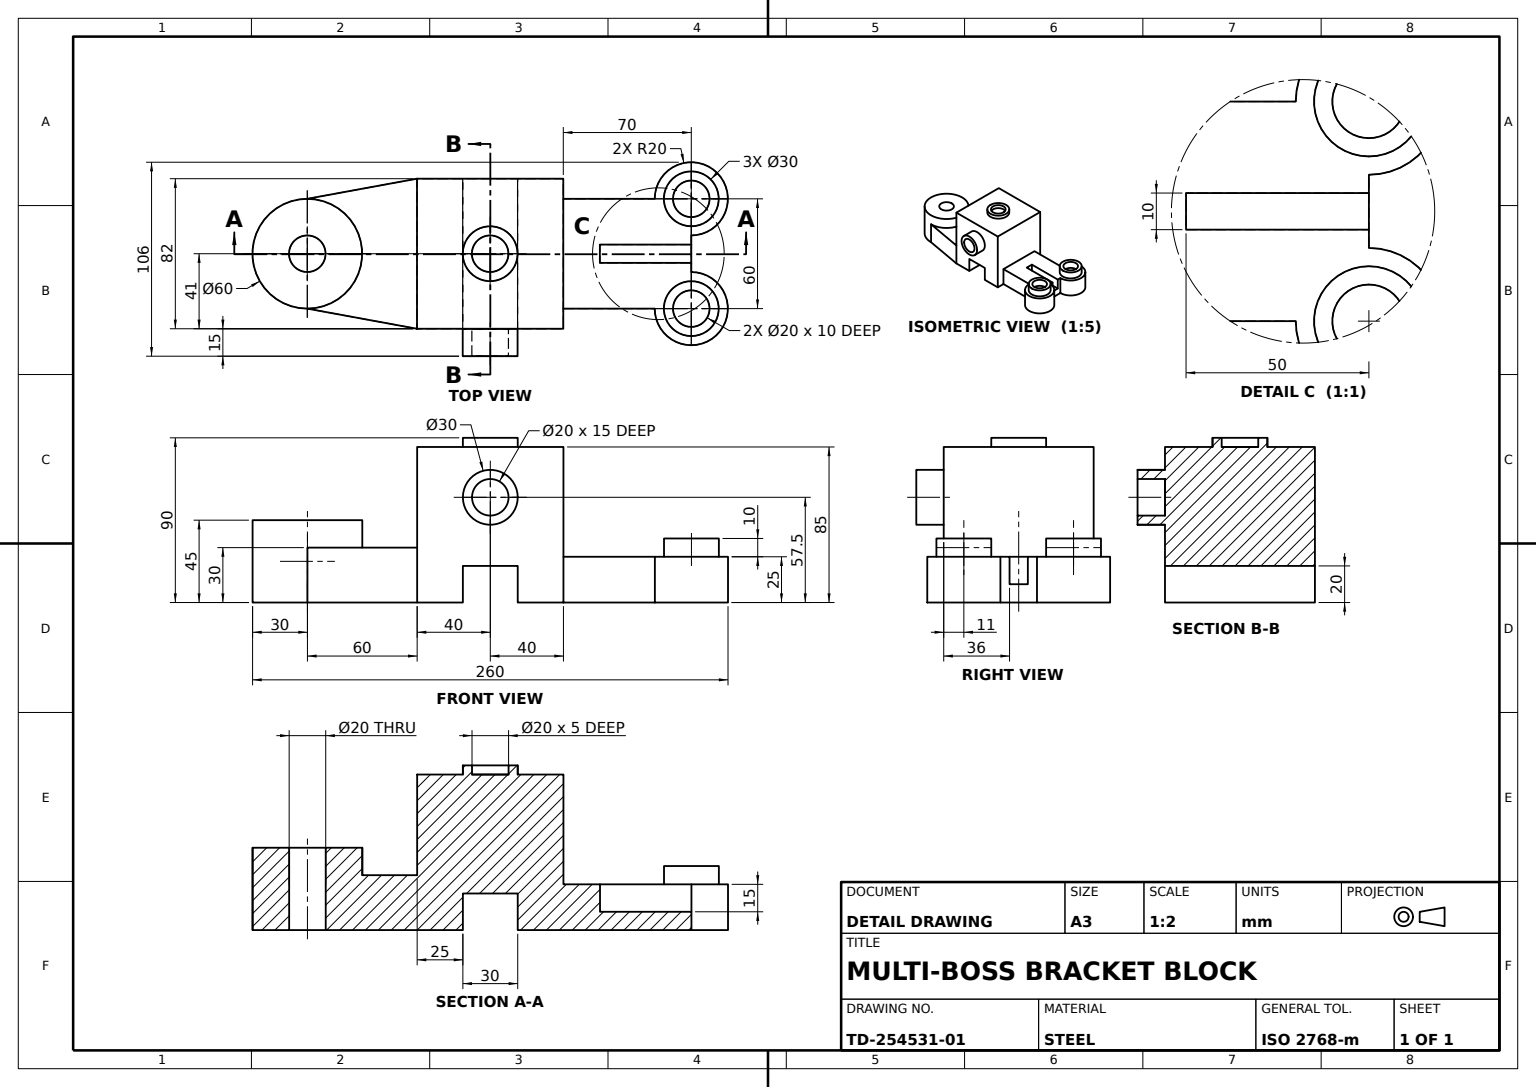
SolidWorks part; units mm, degrees
material "Plain Carbon Steel"
ref_plane "Front Plane" through (0, 0, 0) normal (0, 0, 1) x (1, 0, 0)
ref_plane "Top Plane" through (0, 0, 0) normal (0, 1, 0) x (1, 0, 0)
ref_plane "Right Plane" through (0, 0, 0) normal (1, 0, 0) x (0, 0, -1)
sketch "Main Block Profile" plane through (0, 0, 0) normal (0, 0, 1) x (1, 0, 0)
  line L0 (0, 0) -> (25, 0)
  line L1 (25, 0) -> (25, 20)
  line L2 (25, 20) -> (55, 20)
  line L3 (55, 20) -> (55, 0)
  line L4 (55, 0) -> (80, 0)
  line L5 (80, 0) -> (80, 85)
  line L6 (80, 85) -> (0, 85)
  line L7 (0, 85) -> (0, 0)
  dimension "D1" = 25
  dimension "D2" = 25
  dimension "D3" = 30
  dimension "D4" = 85
  dimension "D5" = 20
extrude "Main Block" add sketch "Main Block Profile" along normal blind 82
ref_plane "Feature Sketch Plane" through (0, 0, 0) normal (0, 1, 0) x (1, 0, 0)
sketch "Side Lug Profile" plane through (0, 0, 0) normal (0, 1, 0) x (1, 0, 0)
  line L0 (0, -41) -> (-60, -41) construction
  line L1 (0, -82) -> (0, 0) construction
  circle A0 centre (-60, -41) radius 10
  circle A1 centre (-60, -41) radius 30
  dimension "D1" = 60
  dimension "D2" = 20
  dimension "D3" = 60
extrude "Side Lug Boss" add sketch "Side Lug Profile" along normal blind 45 separate body
sketch "Gusset Profile" plane through (0, 0, 0) normal (0, 1, 0) x (1, 0, 0)
  line L0 (0, 0) -> (-60, -11)
  line L1 (0, -82) -> (-60, -71)
  line L2 (0, 0) -> (0, -82)
  circle A0 centre (-60, -41) radius 30 construction
  arc A1 (-60, -11) -> (-60, -71) centre (-60, -41) cw
extrude "Gusset Boss" add sketch "Gusset Profile" along normal blind 30
sketch "Mounting Tab Profile" plane through (0, 0, 0) normal (0, 1, 0) x (1, 0, 0)
  line L1 (80, -82) -> (80, 0) construction
  line L3 (80, -11) -> (150, -11)
  line L4 (150, -11) -> (150, -71)
  line L5 (150, -71) -> (80, -71)
  line L6 (80, -71) -> (80, -11)
  dimension "D1" = 70
  dimension "D2" = 60
  dimension "D3" = 11
extrude "Mounting Tab" add sketch "Mounting Tab Profile" along normal blind 25 contours L3 L4 L5 L6
sketch "Tab Eye Profile" plane through (0, 25, 0) normal (0, 1, 0) x (1, 0, 0)
  circle A0 centre (150, -11) radius 20
  circle A1 centre (150, -71) radius 20
  dimension "D1" = 40
  dimension "D2" = 40
extrude "Tab Eye Boss" add sketch "Tab Eye Profile" against normal blind 25
sketch "Tab Ring Profiles" plane through (0, 25, 0) normal (0, 1, 0) x (1, 0, 0)
  circle A0 centre (150, -11) radius 10
  circle A1 centre (150, -11) radius 15
  circle A2 centre (150, -71) radius 10
  circle A3 centre (150, -71) radius 15
  dimension "D1" = 30
  dimension "D2" = 20
  dimension "D3" = 30
  dimension "D4" = 20
extrude "Tab Boss Rings" add sketch "Tab Ring Profiles" along normal blind 10
sketch "Side Hub Ring Profile" plane through (0, 85, 0) normal (0, 1, 0) x (1, 0, 0)
  line L0 (0, -82) -> (0, 0) construction
  line L1 (80, 0) -> (0, 0) construction
  circle A0 centre (40, -41) radius 10
  circle A1 centre (40, -41) radius 15
  dimension "D1" = 20
  dimension "D2" = 30
  dimension "D3" = 40
  dimension "D4" = 41
extrude "Side Hub Ring" add sketch "Side Hub Ring Profile" along normal blind 5
sketch "Top Hub Ring Profile" plane through (0, 0, 82) normal (0, 0, 1) x (1, 0, 0)
  line L0 (0, 30) -> (0, 0) construction
  line L1 (0, 0) -> (25, 0) construction
  circle A0 centre (40, 57.5) radius 10
  circle A1 centre (40, 57.5) radius 15
  dimension "D1" = 30
  dimension "D2" = 20
  dimension "D3" = 40
  dimension "D4" = 57.5
extrude "Top Hub Ring" add sketch "Top Hub Ring Profile" along normal blind 15
sketch "Tab Slot Profile" plane through (0, 25, 0) normal (0, 1, 0) x (1, 0, 0)
  line L0 (150, -41) -> (150, -36)
  line L1 (150, -31) -> (150, -51) construction
  line L2 (150, -36) -> (100, -36)
  line L3 (100, -36) -> (100, -46)
  line L4 (100, -46) -> (150, -46)
  line L5 (150, -46) -> (150, -41)
  line L6 (130, -71) -> (80, -71) construction
  dimension "D1" = 50
  dimension "D2" = 25
extrude "Tab Slot Cut" cut sketch "Tab Slot Profile" against normal blind 15
